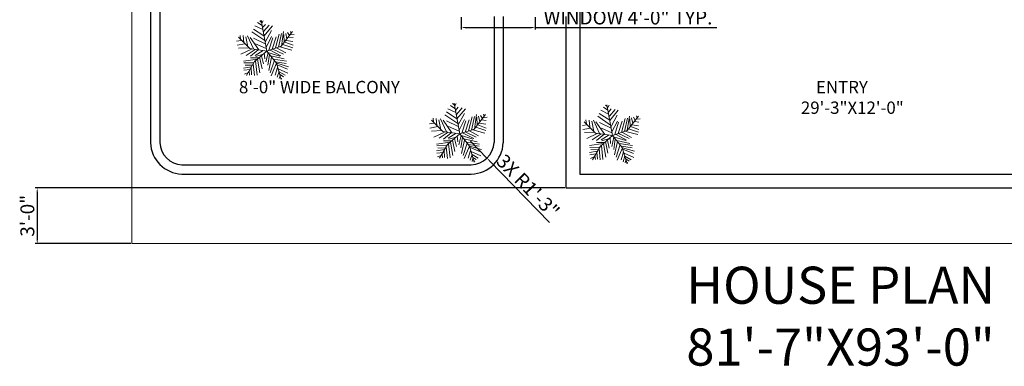
# Model space of a CAD drawing. Units: inches. Extents: x 155 to 1269, y 1260 to 2528.
# Tile 1 of 6: x 155 to 792, y 1260 to 1484. Entities that reach past the tile are written whole.
import ezdxf

# ---------------------------------------------------------------- set-up
doc = ezdxf.new("R2010")
doc.units = ezdxf.units.IN
for name, color, linetype, lineweight in [('A-ANNO-DIMS', 2, 'Continuous', 18), ('A-ANNO-TEXT', 7, 'Continuous', 25), ('A-AREA-IDEN', 7, 'Continuous', 18), ('A-FLOR-EDGE', 7, 'Continuous', 25), ('C-PROP', 8, 'Continuous', 18), ('L-PLNT', 94, 'Continuous', 13)]:
    doc.layers.add(name, color=color, linetype=linetype, lineweight=lineweight)
doc.styles.get("Standard").update_dxf_attribs({"font": 'arial.ttf'})
doc.dimstyles.new('ISO-25', dxfattribs={"dimtxt": 9, "dimasz": 2.5, "dimexe": 1.25, "dimexo": 0.625, "dimtad": 1, "dimlunit": 3, "dimtxsty": 'Standard', "dimcen": 2.5, "dimadec": 0, "dimazin": 0, "dimtfac": 1, "dimtmove": 0, "dimatfit": 3, "dimfxl": 1, "dimarcsym": 0})

# ---------------------------------------------------------------- blocks, each defined once
blk = doc.blocks.new('*U11')
for p, q in [((-10.186, 53.64), (-13.084, 55.962)), ((0, 0), (-10.5, 57)), ((-9.099, 51.782), (-6.563, 55.962)), ((-5.114, 28.097), (-24.676, 40.636)), ((-7.288, 39.707), (-21.778, 46.673)), ((-8.737, 47.138), (-17.069, 52.711)), ((-7.65, 43.423), (-2.578, 49.46)), ((-5.839, 35.992), (4.667, 48.067)), ((-5.114, 27.632), (10.463, 46.673)), ((-2.941, 16.486), (8.652, 37.85)), ((-47.498, 19.737), (-55.83, 18.344)), ((-31.5, 4.5), (-52.5, 25.5)), ((-48.585, 21.131), (-49.309, 29.026)), ((-43.513, 28.561), (-42.427, 15.558)), ((-38.442, 26.239), (-34.819, 7.663)), ((-35.544, 28.097), (-24.314, 3.947)), ((-14.533, 2.09), (-30.834, 25.31)), ((-3.665, 19.273), (-27.574, 35.527)), ((-24.314, 23.917), (-2.941, 13.7)), ((-1.129, 6.734), (9.014, 26.704)), ((3.942, 1.625), (11.187, 24.381)), ((10.101, 3.483), (17.708, 26.239)), ((16.259, 5.805), (23.142, 31.348)), ((22.055, 7.198), (27.489, 32.277)), ((27, 9), (48, 36)), ((27.127, 9.056), (31.112, 35.992)), ((31.836, 30.883), (32.561, 16.486)), ((35.096, 32.741), (37.27, 22.524)), ((36.183, 19.737), (48.137, 17.88)), ((38.719, 34.134), (41.979, 28.561)), ((40.53, 25.775), (48.862, 24.846)), ((43.791, 29.954), (51.036, 30.883)), ((44.153, 36.456), (45.239, 32.741)), ((-40.615, 13.7), (-55.105, 10.913)), ((-33.37, 6.269), (-52.207, 5.34)), ((-28.299, 3.483), (-47.86, -5.805)), ((-21.416, 3.018), (-38.079, -8.128)), ((0, 0), (-31.5, 4.5)), ((-15.982, 2.09), (-30.11, -9.521)), ((0, 0), (-22.5, -19.5)), ((-6.563, 1.161), (-21.416, -8.128)), ((-20.691, 13.7), (-1.129, 4.876)), ((0, 0), (27, 9)), ((0, 0), (18, -22.5)), ((6.478, 1.625), (26.04, -8.592)), ((11.187, 3.483), (30.749, -5.805)), ((18.07, 5.805), (35.096, -3.483)), ((24.229, 7.663), (46.688, 1.625)), ((29.662, 12.307), (48.137, 6.269)), ((33.285, 16.486), (48.862, 10.913)), ((-17.431, -15.094), (-42.789, -18.809)), ((-15.257, -12.772), (-30.11, -12.772)), ((-6.563, -5.805), (-19.967, -9.985)), ((-17.069, -15.094), (-12.721, -40.172)), ((-13.446, -11.378), (-8.737, -32.741)), ((-9.461, -8.592), (-6.201, -23.453)), ((-4.752, -3.483), (-3.665, -14.629)), ((2.493, -3.019), (-1.491, -20.202)), ((1.769, -2.555), (24.229, -9.521)), ((5.029, -6.27), (2.131, -25.775)), ((9.014, -11.378), (3.58, -35.992)), ((14.085, -16.951), (6.478, -40.172)), ((7.565, -9.056), (32.198, -14.629)), ((12.274, -15.094), (36.907, -18.809)), ((-28.299, -29.026), (-42.789, -31.348)), ((-24.314, -21.596), (-42.427, -22.06)), ((-30.834, -34.135), (-42.427, -35.528)), ((-26.849, -26.24), (-40.253, -25.775)), ((-22.5, -19.5), (-37.5, -45)), ((-29.023, -30.884), (-27.936, -43.887)), ((-25.038, -23.918), (-22.865, -45.281)), ((-20.691, -18.345), (-17.793, -44.352)), ((18.07, -22.524), (8.289, -45.745)), ((20.244, -30.419), (15.897, -44.816)), ((16.259, -19.738), (36.183, -22.989)), ((18, -22.5), (27, -52.5)), ((18.433, -22.524), (40.53, -29.026)), ((19.157, -25.311), (38.719, -33.206)), ((21.331, -32.741), (39.081, -40.636)), ((-34.457, -39.708), (-40.978, -42.494)), ((-32.646, -36.921), (-31.921, -44.352)), ((22.78, -37.85), (19.519, -48.532)), ((22.78, -38.314), (34.372, -44.816)), ((24.591, -45.745), (23.142, -50.854)), ((24.591, -43.423), (30.749, -47.603)), ((26.764, -49.925), (28.213, -50.854))]:
    blk.add_line(p, q)
blk = doc.blocks.new('*D34')
at = {"layer": 'A-ANNO-DIMS', "color": 0, "lineweight": -2, "transparency": 16777216}
for p, q in [((440.63, 1485.56), (440.63, 1477.73)), ((488.63, 1485.56), (488.63, 1477.73)), ((443.13, 1478.98), (486.13, 1478.98)), ((488.63, 1478.98), (606.27, 1478.98))]:
    blk.add_line(p, q, dxfattribs=at)
at = {"layer": 'A-ANNO-DIMS', "color": 0, "transparency": 16777216}
for points in [[(443.13, 1479.4), (443.13, 1478.56), (440.63, 1478.98)], [(486.13, 1479.4), (486.13, 1478.56), (488.63, 1478.98)]]:
    blk.add_solid(points, dxfattribs=at)
at = {"layer": 'Defpoints', "color": 0, "transparency": 16777216}
for p in [(440.63, 1486.18), (488.63, 1486.18), (488.63, 1478.98)]:
    blk.add_point(p, dxfattribs=at)
at = {"layer": 'A-ANNO-DIMS', "color": 0, "transparency": 16777216, "insert": (548.7, 1484.26), "char_height": 9, "attachment_point": 5}
blk.add_mtext('WINDOW 4\'-0" TYP.', dxfattribs=at)
blk = doc.blocks.new('*D36')
at = {"layer": 'A-ANNO-DIMS', "color": 0, "lineweight": -2, "transparency": 16777216}
for p, q in [((373.64, 1500.1), (373.64, 1497.76)), ((376.14, 1499.01), (382.53, 1499.01)), ((385.03, 1500.1), (385.03, 1497.76)), ((385.03, 1499.01), (527.79, 1499.01))]:
    blk.add_line(p, q, dxfattribs=at)
at = {"layer": 'A-ANNO-DIMS', "color": 0, "transparency": 16777216}
for points in [[(376.14, 1499.43), (376.14, 1498.6), (373.64, 1499.01)], [(382.53, 1499.43), (382.53, 1498.6), (385.03, 1499.01)]]:
    blk.add_solid(points, dxfattribs=at)
at = {"layer": 'Defpoints', "color": 0, "transparency": 16777216}
for p in [(373.64, 1500.72), (385.03, 1500.72), (385.03, 1499.01)]:
    blk.add_point(p, dxfattribs=at)
at = {"layer": 'A-ANNO-DIMS', "color": 0, "transparency": 16777216, "insert": (457.66, 1504.29), "char_height": 9, "attachment_point": 5}
blk.add_mtext('BURNER 0\'-11 1/2" TYP.', dxfattribs=at)
blk = doc.blocks.new('*D44')
at = {"layer": 'A-ANNO-DIMS', "color": 0, "lineweight": -2, "transparency": 16777216}
for p, q in [((507.77, 1375.18), (164.8, 1375.18)), ((166.05, 1372.68), (166.05, 1341.68)), ((226.77, 1339.18), (164.8, 1339.18))]:
    blk.add_line(p, q, dxfattribs=at)
at = {"layer": 'A-ANNO-DIMS', "color": 0, "transparency": 16777216}
for points in [[(165.63, 1372.68), (166.46, 1372.68), (166.05, 1375.18)], [(165.63, 1341.68), (166.46, 1341.68), (166.05, 1339.18)]]:
    blk.add_solid(points, dxfattribs=at)
at = {"layer": 'Defpoints', "color": 0, "transparency": 16777216}
for p in [(508.4, 1375.18), (166.05, 1339.18), (227.4, 1339.18)]:
    blk.add_point(p, dxfattribs=at)
at = {"layer": 'A-ANNO-DIMS', "color": 0, "transparency": 16777216, "insert": (160.82, 1357.18), "char_height": 9, "attachment_point": 5, "rotation": 90}
blk.add_mtext('3\'-0"', dxfattribs=at)
blk = doc.blocks.new('*D57')
at = {"layer": 'A-ANNO-DIMS', "color": 0, "lineweight": -2, "transparency": 16777216}
for p, q in [((446.69, 1405.41), (457.32, 1394.5)), ((497.89, 1352.88), (459.07, 1392.71))]:
    blk.add_line(p, q, dxfattribs=at)
at = {"layer": 'A-ANNO-DIMS', "color": 0, "transparency": 16777216}
blk.add_solid([(459.36, 1393), (458.77, 1392.42), (457.32, 1394.5)], dxfattribs=at)
at = {"layer": 'Defpoints', "color": 0, "transparency": 16777216}
for p in [(446.69, 1405.41), (457.32, 1394.5)]:
    blk.add_point(p, dxfattribs=at)
at = {"layer": 'A-ANNO-DIMS', "color": 0, "transparency": 16777216, "insert": (483.09, 1375.55), "char_height": 9, "attachment_point": 5, "rotation": 314.26583}
blk.add_mtext('3X R1\'-3"', dxfattribs=at)

msp = doc.modelspace()

# ---------------------------------------------------------------- linework, layer by layer
at = {"layer": 'A-FLOR-EDGE'}
for p, q in [((239.397, 1713.12), (239.397, 1404.446)), ((245.397, 1712.609), (245.397, 1404.556)), ((517.397, 1525.181), (517.397, 1384.181)), ((461.899, 1486.181), (461.899, 1404.585)), ((467.899, 1486.181), (467.899, 1404.435)), ((508.397, 1486.181), (508.397, 1384.181)), ((259.599, 1384.181), (447.201, 1384.181)), ((259.719, 1390.181), (447.122, 1390.181)), ((508.397, 1384.181), (508.397, 1375.181)), ((517.397, 1384.181), (868.397, 1384.181)), ((508.397, 1375.181), (877.397, 1375.181))]:
    msp.add_line(p, q, dxfattribs=at)
for centre, radius, start, end in [((260.376, 1405.157), 20.991, 181.941445, 267.878551), ((260.376, 1405.157), 14.991, 182.2974, 267.489584), ((446.686, 1405.41), 15.235, 271.638477, 356.895339), ((446.686, 1405.41), 21.235, 271.387815, 357.37037)]:
    msp.add_arc(centre, radius, start, end, dxfattribs=at)
at = {"layer": 'C-PROP'}
for p, q in [((227.397, 2455.181), (227.397, 1339.181)), ((227.397, 1339.181), (1206.397, 1339.181))]:
    msp.add_line(p, q, dxfattribs=at)

# ---------------------------------------------------------------- block references
at = {"layer": 'L-PLNT', "xscale": 0.3495173552522817, "yscale": 0.3495173552522817, "zscale": 0.3495173552522817}
for p in [(314.697, 1463.73), (439.678, 1410.15), (538.697, 1409.112)]:
    msp.add_blockref('*U11', p, dxfattribs=at)

# ---------------------------------------------------------------- texts
at = {"layer": 'A-ANNO-TEXT', "insert": (586.462, 1324.251), "char_height": 24, "attachment_point": 1}
msp.add_mtext_dynamic_manual_height_columns('HOUSE PLAN \\P81\'-7"X93\'-0"', width=232.89447, gutter_width=12.5, heights=[0], dxfattribs=at)
at = {"layer": 'A-AREA-IDEN', "char_height": 8, "attachment_point": 1}
for s, width, insert in [('8\'-0" WIDE BALCONY', 110.88305, (296.714, 1444.437)), ('    ENTRY \\P29\'-3"X12\'-0"', 65.0847, (660.668, 1444.437))]:
    msp.add_mtext_dynamic_manual_height_columns(s, width=width, gutter_width=12.5, heights=[0], dxfattribs=dict(at, insert=insert))

# ---------------------------------------------------------------- dimensions: what is measured, and where the dimension line sits
at = {"layer": 'A-ANNO-DIMS'}
for base, p1, p2, text, picture, middle in [((385.03, 1499.015), (373.642, 1500.723), (385.03, 1500.723), 'BURNER <> TYP.', '*D36', (457.659, 1504.293)), ((488.631, 1478.981), (440.631, 1486.181), (488.631, 1486.181), 'WINDOW <> TYP.', '*D34', (548.7, 1484.262))]:
    dim = msp.add_linear_dim(base=base, p1=p1, p2=p2, text=text, dimstyle='ISO-25', override={"dimdec": 1, "dimlfac": 1, "dimrnd": 0, "dimzin": 1, "dimdsep": 46, "dimlunit": 4, "dimfrac": 2}, dxfattribs=at)
    dim.commit()
    dim.dimension.update_dxf_attribs({"geometry": picture, "text_midpoint": middle})
dim = msp.add_radius_dim(center=(446.686, 1405.41), mpoint=(457.32, 1394.5), text='3X <>', dimstyle='ISO-25', override={"dimdec": 1, "dimlfac": 1, "dimrnd": 0, "dimzin": 1, "dimdsep": 46, "dimlunit": 4, "dimfrac": 2}, dxfattribs=at)
dim.commit()
dim.dimension.update_dxf_attribs({"geometry": '*D57', "text_midpoint": (483.089, 1375.545)})
dim = msp.add_linear_dim(base=(166.047, 1339.181), p1=(508.397, 1375.181), p2=(227.397, 1339.181), angle=90, dimstyle='ISO-25', override={"dimdec": 1, "dimlfac": 1, "dimrnd": 0, "dimzin": 1, "dimdsep": 46, "dimlunit": 4, "dimfrac": 2}, dxfattribs=at)
dim.commit()
dim.dimension.update_dxf_attribs({"geometry": '*D44', "text_midpoint": (160.824, 1357.181)})

doc.saveas('drawing.dxf')
